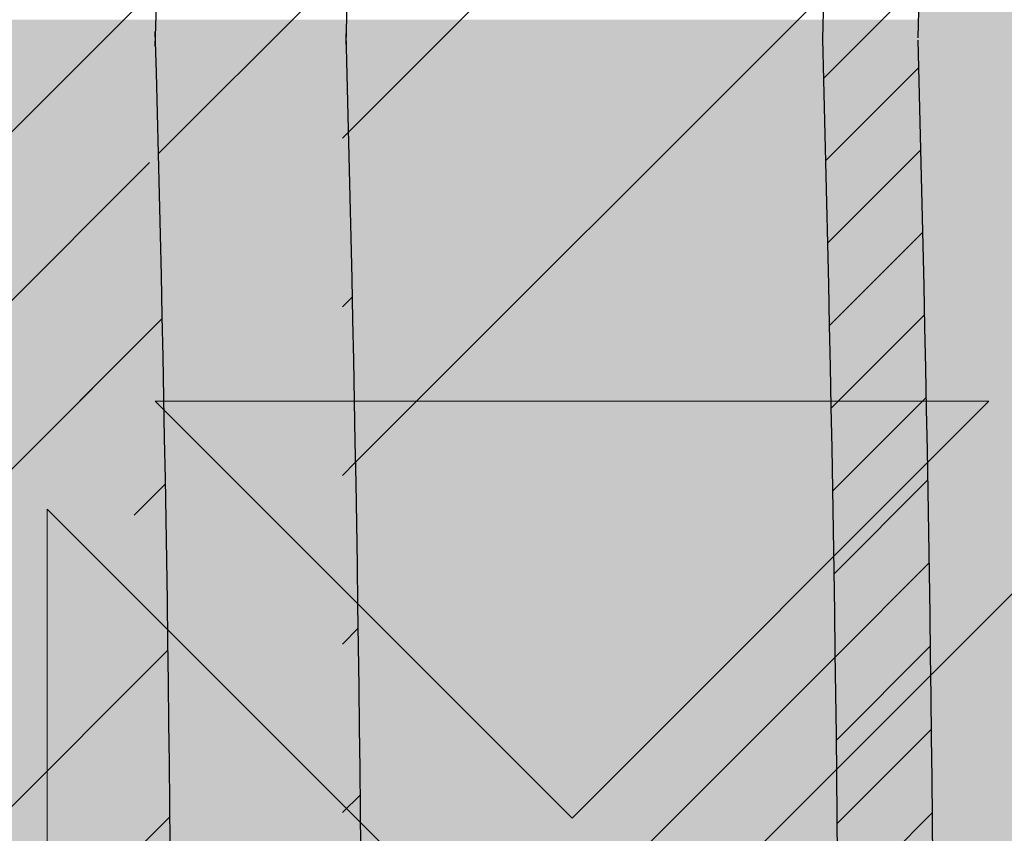
# Model space of a CAD drawing. Units: inches. Extents: x 844 to 2234, y 346 to 1084.
# Tile 11 of 93: x 1124.948 to 1126.594, y 694.861 to 696.22. Entities that reach past the tile are written whole.
import ezdxf

# ---------------------------------------------------------------- set-up
doc = ezdxf.new("R2010")
doc.units = ezdxf.units.IN
doc.header["$MEASUREMENT"] = 0
for name, color, linetype, lineweight in [('A-ANNO-DIMS', 2, 'Continuous', 18), ('furniture', 8, 'Continuous', 18), ('RA-AP-01$0$INT', 35, 'Continuous', 5)]:
    doc.layers.add(name, color=color, linetype=linetype, lineweight=lineweight)
doc.layers.add('RA-AP-01$0$FURN', color=3, linetype='Continuous')
doc.layers.add('RA-AP-01$0$WOOD', color=64, linetype='Continuous')
doc.styles.get("Standard").update_dxf_attribs({"font": 'arial.ttf'})
doc.dimstyles.get("Standard").update_dxf_attribs({"dimtxt": 6, "dimasz": 3, "dimexe": 0.18, "dimexo": 0.0625, "dimgap": 0.09, "dimtad": 0, "dimtih": 1, "dimtoh": 1, "dimdec": 1, "dimzin": 0, "dimdsep": 46, "dimlunit": 3, "dimtxsty": 'Standard', "dimblk": 'ARCHTICK', "dimcen": 0.09, "dimadec": 0, "dimazin": 0, "dimtfac": 1, "dimtdec": 1, "dimtofl": 0, "dimtmove": 0, "dimatfit": 3, "dimfxl": 1, "dimtolj": 1, "dimtzin": 0, "dimarcsym": 0})

# ---------------------------------------------------------------- blocks, each defined once
blk = doc.blocks.new('A$C18D01794')
at = {"layer": 'RA-AP-01$0$INT'}
h = blk.add_hatch(color=256, dxfattribs=at)
h.paths.add_polyline_path([(4.585917135068449, -6.356712009588271), (4.555206456959269, -6.35671200958746), (4.555206456959137, -6.387422687716308), (4.874495778835233, -6.706712009592356), (4.90520645695423, -6.676001331474049)])
h.paths.add_polyline_path([(5.255206456948813, -6.387422687716306), (5.255206456948682, -6.356712009605972), (5.224495778822613, -6.356712009605161), (4.905206456953498, -6.676001331474273), (4.935917135072151, -6.706712009592924)])
h.paths.add_polyline_path([(4.935917135072559, -6.706712009592068), (4.905206456953564, -6.737422687710376), (5.255206456951813, -7.087422687708613), (5.255206456951549, -7.026001331471008)])
h.paths.add_polyline_path([(4.555206456956399, -7.026001331471013), (4.555206456956134, -7.087422687708616), (4.905206456953821, -6.737422687710943), (4.874495778835166, -6.70671200959229)])
h = blk.add_hatch(color=256, dxfattribs=at)
h.paths.add_polyline_path([(4.585917135068448, -6.356712009588273), (4.614201406330596, -6.356712009589021), (4.668846067270487, -6.411356670531338), (4.723490728212344, -6.356712009591912), (4.771774999457151, -6.35671200959319), (4.826419660396886, -6.411356670535356), (4.862780050090322, -6.374996280843536), (4.844495778842715, -6.356712009595112), (4.862780050090411, -6.356712009595595), (4.905206456960182, -6.399138416468211), (4.947632863832445, -6.356712009597838), (4.965917135079675, -6.356712009598322), (4.947632863831759, -6.374996280845421), (4.983993253523576, -6.411356670538857), (5.038637914464627, -6.356712009600247), (5.08692218571208, -6.356712009601523), (5.141566846649976, -6.411356670541852), (5.196211507589851, -6.356712009604411), (5.224495778822615, -6.356712009605161), (4.905206456953975, -6.676001331473793)])
h.paths.add_polyline_path([(4.895206456956031, -6.637717060225675), (4.895206456958921, -6.528427738347902), (4.840561796018589, -6.583072399285802)], flags=16)
h.paths.add_polyline_path([(4.915206456955638, -6.637717060226121), (4.969851117895509, -6.583072399288678), (4.915206456957609, -6.528427738348344)], flags=16)
h.paths.add_polyline_path([(4.826419660395175, -6.568930263661755), (4.881064321335613, -6.514285602723745), (4.771774999456703, -6.514285602720857)], flags=16)
h.paths.add_polyline_path([(4.983993253519558, -6.568930263665262), (5.038637914460456, -6.514285602726792), (4.929348592581548, -6.514285602724816)], flags=16)
h.paths.add_polyline_path([(4.881064321336025, -6.494285602723742), (4.826419660397532, -6.439640941782821), (4.771774999457062, -6.494285602720859)], flags=16)
h.paths.add_polyline_path([(4.929348592582019, -6.494285602724817), (5.038637914460982, -6.494285602726792), (4.983993253522945, -6.439640941786327)], flags=16)
h.paths.add_polyline_path([(4.895206456960191, -6.480143467100443), (4.895206456962115, -6.407422687715913), (4.876922185715016, -6.389138416467584), (4.840561796021581, -6.425498806159401)], flags=16)
h.paths.add_polyline_path([(4.915206456958487, -6.480143467100889), (4.969851117899527, -6.425498806162279), (4.933490728206909, -6.389138416468043), (4.9152064569598, -6.40742268771434)], flags=16)
h.paths.add_polyline_path([(4.757632863832376, -6.480143467096812), (4.812277524772842, -6.425498806158772), (4.757632863834348, -6.370854145217844)], flags=16)
h.paths.add_polyline_path([(4.737632863832376, -6.480143467096286), (4.737632863834348, -6.370854145217375), (4.682988202893906, -6.425498806155385)], flags=16)
h.paths.add_polyline_path([(5.05278005008503, -6.480143467103376), (5.052780050087917, -6.370854145224413), (4.998135389146995, -6.425498806162908)], flags=16)
h.paths.add_polyline_path([(5.072780050085024, -6.480143467103744), (5.127424711025931, -6.42549880616527), (5.072780050087916, -6.370854145224832)], flags=16)
h.paths.add_polyline_path([(4.935917135072783, -6.706712009592292), (5.255206456948811, -6.387422687716309), (5.255206456948932, -6.415706958964177), (5.200561796010279, -6.470351619902839), (5.255206456949403, -6.524996280841948), (5.25520645694961, -6.5732805520894), (5.200561796009787, -6.627925213029239), (5.236922185702417, -6.664285602721864), (5.255206456949919, -6.646001331474357), (5.255206456949998, -6.664285602721898), (5.212780050078687, -6.706712009592262), (5.25520645695036, -6.749138416463932), (5.255206456950438, -6.767422687711313), (5.236922185702424, -6.749138416463297), (5.200561796009796, -6.785498806155928), (5.255206456950753, -6.840143467096874), (5.25520645695096, -6.888427738341682), (5.200561796010322, -6.943072399282328), (5.255206456951428, -6.997717060223427), (5.255206456951547, -7.026001331471006)])
h.paths.add_polyline_path([(5.042988202883395, -6.785498806155427), (5.097632863823085, -6.840143467095101), (5.097632863822622, -6.730854145216193)], flags=16)
h.paths.add_polyline_path([(5.028846067259663, -6.771356670531693), (5.083490728198774, -6.716712009592573), (4.974201406321001, -6.716712009593042)], flags=16)
h.paths.add_polyline_path([(5.117632863823087, -6.840143467095186), (5.172277524762331, -6.785498806155926), (5.11763286382262, -6.730854145216225)], flags=16)
h.paths.add_polyline_path([(5.08349072819877, -6.696712009593886), (5.028846067259652, -6.642067348654775), (4.974201406320998, -6.696712009593438)], flags=16)
h.paths.add_polyline_path([(5.131774999446817, -6.854285602718917), (5.186419660386065, -6.799640941779662), (5.241064321325782, -6.854285602719365)], flags=17)
h.paths.add_polyline_path([(5.131774999446228, -6.716712009592374), (5.186419660386065, -6.771356670532194), (5.222780050079488, -6.734996280838764), (5.204495778832781, -6.716712009592063)], flags=16)
h.paths.add_polyline_path([(5.097632863822613, -6.682569873970264), (5.097632863823061, -6.573280552091354), (5.042988202883383, -6.627925213031044)], flags=16)
h.paths.add_polyline_path([(5.131774999446899, -6.874285602718915), (5.241064321325809, -6.874285602719364), (5.186419660386591, -6.928930263658598)], flags=17)
h.paths.add_polyline_path([(5.131774999446226, -6.696712009594078), (5.204495778830767, -6.696712009594374), (5.22278005007868, -6.67842773834687), (5.186419660386049, -6.642067348654249)], flags=16)
h.paths.add_polyline_path([(5.11763286382262, -6.682569873970225), (5.17227752476232, -6.627925213030515), (5.117632863823064, -6.573280552091267)], flags=16)
h.paths.add_polyline_path([(5.186419660386069, -6.613783077405491), (5.241064321325754, -6.559138416465795), (5.131774999446791, -6.559138416466263)], flags=16)
h.paths.add_polyline_path([(5.131774999446872, -6.539138416466263), (5.24106432132578, -6.539138416465794), (5.186419660386554, -6.484493755526573)], flags=16)
h.paths.add_polyline_path([(5.255206456951811, -7.08742268770861), (5.255206456951895, -7.106712009588038), (4.555206456956052, -7.106712009588038), (4.555206456956136, -7.087422687708617), (4.905206456953973, -6.737422687710788)])
h.paths.add_polyline_path([(4.983993253513404, -6.8444937555241), (4.92934859257295, -6.899138416462108), (5.03863791445186, -6.899138416465014)], flags=16)
h.paths.add_polyline_path([(4.969851117889988, -6.83035161990006), (4.915206456952556, -6.775706958960171), (4.915206456949648, -6.884996280837944)], flags=16)
h.paths.add_polyline_path([(4.929348592572535, -6.919138416462105), (4.983993253511019, -6.973783077403037), (5.038637914451496, -6.919138416465012)], flags=16)
h.paths.add_polyline_path([(5.052780050074912, -6.93328055208906), (4.998135389134438, -6.987925213027088), (5.052780050072919, -7.042569873968025)], flags=16)
h.paths.add_polyline_path([(5.07278005007491, -6.933280552089588), (5.072780050072918, -7.042569873968497), (5.127424711013374, -6.987925213030498)], flags=16)
h.paths.add_polyline_path([(4.89520645695295, -6.775706958959721), (4.840561796013067, -6.830351619897157), (4.895206456950961, -6.884996280837494)], flags=16)
h.paths.add_polyline_path([(4.915206456948365, -6.933280552085403), (4.915206456946434, -7.006001331471951), (4.933490728192729, -7.024285602719066), (4.969851117886972, -6.987925213026453)], flags=16)
h.paths.add_polyline_path([(4.881064321327021, -6.899138416461022), (4.82641966038902, -6.84449375552057), (4.771774999448108, -6.899138416459029)], flags=16)
h.paths.add_polyline_path([(4.895206456950073, -6.933280552084951), (4.840561796009022, -6.987925213023558), (4.876922185700835, -7.024285602716997), (4.895206456948749, -7.006001331469487)], flags=16)
h.paths.add_polyline_path([(4.983993253510392, -7.0020673486505), (4.947632863816944, -7.038427738342319), (4.965917135064043, -7.05671200959023), (5.038637914448995, -7.056712009591555)], flags=16)
h.paths.add_polyline_path([(4.881064321326543, -6.91913841646102), (4.771774999447578, -6.919138416459031), (4.826419660385607, -6.973783077399508)], flags=16)
h.paths.add_polyline_path([(4.905206456946447, -7.014285602717636), (4.862780050074785, -7.056712009588352), (4.947632863816685, -7.056712009589775)], flags=16)
h.paths.add_polyline_path([(5.14156684663679, -7.002067348654549), (5.086922185696452, -7.056712009592438), (5.196211507574223, -7.056712009594425)], flags=16)
h.paths.add_polyline_path([(4.8264196603837, -7.002067348646972), (4.771774999442643, -7.056712009585575), (4.8444957788276, -7.056712009587508), (4.862780050075511, -7.038427738340416)], flags=16)
h.paths.add_polyline_path([(4.812277524760289, -6.98792521302292), (4.757632863822258, -6.933280552082447), (4.757632863819352, -7.042569873961408)], flags=16)
h.paths.add_polyline_path([(4.73763286382226, -6.933280552082079), (4.682988202881349, -6.987925213020536), (4.737632863819352, -7.04256987396099)], flags=16)
h.paths.add_polyline_path([(4.723490728195188, -7.056712009584289), (4.668846067257299, -7.002067348643949), (4.614201406317417, -7.056712009581383)], flags=16)
h.paths.add_polyline_path([(4.597632863829262, -6.706712009592262), (4.555206456957951, -6.664285602721896), (4.555206456958029, -6.646001331474357), (4.573490728205535, -6.664285602721864), (4.609851117898167, -6.627925213029238), (4.555206456958338, -6.573280552089402), (4.555206456958546, -6.524996280841952), (4.60985111789767, -6.470351619902839), (4.555206456959015, -6.415706958964177), (4.555206456959138, -6.387422687716309), (4.874495778835167, -6.70671200959229), (4.5552064569564, -7.026001331471015), (4.555206456956523, -6.997717060223433), (4.609851117897629, -6.94307239928233), (4.555206456956988, -6.888427738341681), (4.555206456957198, -6.840143467096881), (4.609851117898153, -6.78549880615593), (4.573490728205528, -6.749138416463297), (4.555206456957507, -6.76742268771132), (4.555206456957585, -6.749138416463933)])
h.paths.add_polyline_path([(4.712780050085332, -6.730854145216195), (4.712780050084863, -6.840143467095105), (4.767424711024555, -6.785498806155427)], flags=16)
h.paths.add_polyline_path([(4.726922185709173, -6.716712009592573), (4.781566846648288, -6.771356670531693), (4.836211507586949, -6.716712009593043)], flags=16)
h.paths.add_polyline_path([(4.692780050085327, -6.730854145216225), (4.638135389145619, -6.785498806155928), (4.692780050084865, -6.840143467095185)], flags=16)
h.paths.add_polyline_path([(4.726922185709182, -6.696712009593886), (4.836211507586949, -6.696712009593436), (4.7815668466483, -6.642067348654773)], flags=16)
h.paths.add_polyline_path([(4.678637914461726, -6.71671200959237), (4.605917135075169, -6.716712009592063), (4.587632863828464, -6.734996280838766), (4.623993253521887, -6.771356670532195)], flags=16)
h.paths.add_polyline_path([(4.712780050085336, -6.68256987397026), (4.767424711024568, -6.627925213031042), (4.71278005008489, -6.573280552091352)], flags=16)
h.paths.add_polyline_path([(4.678637914461726, -6.696712009594076), (4.623993253521899, -6.642067348654247), (4.587632863829271, -6.67842773834687), (4.605917135077185, -6.696712009594376)], flags=16)
h.paths.add_polyline_path([(4.692780050085336, -6.682569873970228), (4.692780050084889, -6.573280552091267), (4.638135389145632, -6.627925213030515)], flags=16)
h.paths.add_polyline_path([(4.623993253521885, -6.799640941779662), (4.678637914461131, -6.854285602718915), (4.56934859258217, -6.854285602719365)], flags=17)
h.paths.add_polyline_path([(4.623993253521901, -6.613783077405509), (4.678637914461158, -6.559138416466263), (4.569348592582195, -6.559138416465795)], flags=16)
h.paths.add_polyline_path([(4.678637914461051, -6.874285602718915), (4.623993253521361, -6.928930263658598), (4.569348592582143, -6.874285602719364)], flags=17)
h.paths.add_polyline_path([(4.678637914461076, -6.539138416466263), (4.623993253521399, -6.484493755526573), (4.569348592582167, -6.539138416465796)], flags=16)
h = blk.add_hatch(color=256, dxfattribs=at)
h.paths.add_polyline_path([(4.895206456952951, -6.77570695895972), (4.840561796013068, -6.830351619897156), (4.895206456950958, -6.884996280837495)])
h.paths.add_polyline_path([(4.915206456949649, -6.884996280837942), (4.969851117889987, -6.830351619900054), (4.915206456952556, -6.775706958960171)])
h.paths.add_polyline_path([(5.038637914451862, -6.899138416465013), (4.983993253513403, -6.8444937555241), (4.929348592572953, -6.899138416462106)])
h.paths.add_polyline_path([(4.929348592572535, -6.919138416462105), (4.983993253511018, -6.973783077403037), (5.038637914451497, -6.919138416465012)])
h.paths.add_polyline_path([(4.915206456948366, -6.933280552085397), (4.915206456946433, -7.006001331471951), (4.93349072819273, -7.024285602719068), (4.969851117886972, -6.987925213026454)])
h.paths.add_polyline_path([(5.038637914448995, -7.056712009591553), (4.983993253510389, -7.002067348650502), (4.947632863816946, -7.038427738342318), (4.965917135064043, -7.05671200959023)])
h.paths.add_polyline_path([(5.05278005007292, -7.042569873968023), (5.05278005007491, -6.933280552089059), (4.998135389134438, -6.987925213027088)])
h.paths.add_polyline_path([(5.07278005007292, -7.042569873968496), (5.127424711013374, -6.987925213030498), (5.072780050074909, -6.933280552089588)])
h.paths.add_polyline_path([(5.141566846636789, -7.002067348654547), (5.086922185696449, -7.056712009592438), (5.196211507574223, -7.056712009594425)])
h.paths.add_polyline_path([(4.947632863816688, -7.056712009589774), (4.905206456946449, -7.014285602717634), (4.862780050074784, -7.056712009588353)])
h.paths.add_polyline_path([(4.840561796009025, -6.987925213023556), (4.876922185700834, -7.024285602716997), (4.895206456948747, -7.006001331469488), (4.895206456950075, -6.933280552084953)])
h.paths.add_polyline_path([(4.88106432132654, -6.919138416461021), (4.771774999447577, -6.919138416459031), (4.826419660385606, -6.973783077399508)])
h.paths.add_polyline_path([(4.881064321327019, -6.899138416461022), (4.826419660389019, -6.844493755520571), (4.771774999448108, -6.89913841645903)])
h.paths.add_polyline_path([(4.757632863819352, -7.042569873961409), (4.812277524760284, -6.987925213022922), (4.757632863822259, -6.933280552082447)])
h.paths.add_polyline_path([(4.8264196603837, -7.002067348646974), (4.771774999442646, -7.056712009585575), (4.844495778827599, -7.05671200958751), (4.862780050075512, -7.038427738340417)])
h.paths.add_polyline_path([(4.737632863819352, -7.042569873960988), (4.737632863822258, -6.933280552082078), (4.682988202881349, -6.987925213020538)])
h.paths.add_polyline_path([(4.668846067257299, -7.002067348643952), (4.61420140631742, -7.056712009581384), (4.723490728195189, -7.056712009584292)])
for p, q in [((4.905206456953975, -6.737422687710788), (5.255206456951811, -7.087422687708611)), ((5.07278005007491, -6.933280552089588), (5.07278005007292, -7.042569873968497)), ((5.07278005007292, -7.042569873968497), (5.127424711013374, -6.987925213030498)), ((5.086922185696454, -7.056712009592434), (5.141566846636789, -7.002067348654547)), ((5.196211507574223, -7.056712009594425), (5.141566846636789, -7.002067348654547)), ((5.086922185696452, -7.056712009592438), (5.196211507574223, -7.056712009594425))]:
    blk.add_line(p, q, dxfattribs=at)
blk = doc.blocks.new('A$C32926AE1')
at = {"layer": 'RA-AP-01$0$FURN'}
h = blk.add_hatch(dxfattribs=at)
h.set_pattern_fill('ANSI31', color=256, scale=0.1, style=0)
h.set_pattern_definition([(45, (0, 0), (-0.0088388347648318, 0.0088388347648318), [])])
edge = h.paths.add_edge_path(flags=16)
edge.add_arc((4.904771284329206, 4.246793130718756), 0.2603971832811541, 75.22398030683196, 104.7760196931204)
edge.add_arc((4.904771284329206, 4.246793130718756), 0.2603971832811541, 75.223980306832, 104.77601969312039, ccw=False)
edge = h.paths.add_edge_path(flags=16)
edge.add_arc((4.904771284329206, 4.067062675376612), 0.2603971832811541, 255.2239803068796, 284.776019693168)
edge.add_arc((4.904771284329206, 4.067062675376612), 0.2603971832811541, 255.22398030687958, 284.77601969316805, ccw=False)
edge = h.paths.add_edge_path(flags=0)
edge.add_arc((4.904771284329206, 4.067062675376612), 0.2603971832811541, 255.2239803068796, 284.776019693168)
edge.add_arc((4.904771284329206, 4.067062675376612), 0.2603971832811541, 255.22398030687958, 284.77601969316805, ccw=False)
edge = h.paths.add_edge_path(flags=0)
edge.add_arc((4.904771284329206, 4.067062675376612), 0.2603971832811541, 255.2239803068796, 284.776019693168)
edge.add_arc((4.904771284329206, 4.067062675376612), 0.2603971832811541, 255.22398030687958, 284.77601969316805, ccw=False)
edge = h.paths.add_edge_path()
edge.add_arc((4.604388392048174, 4.588829985554312), 0.1599999999999918, 342.3781640246255, 354.4317409793762)
edge.add_arc((5.090145208887507, 4.43216705527679), 0.3503971832811637, 162.0091218307731, 180.3186872093483)
edge.add_arc((5.205154176610243, 4.588829985554953), 0.1599999999999917, 185.5682590208461, 197.6218359767349)
edge.add_arc((4.904771284329229, 4.246793130718735), 0.3503971832811761, 72.00912183053516, 107.9908781690354)
edge.add_arc((9.535952835716557, 4.28682295566602), 4.798342501046485, 178.2875002453811, 181.5576802719453)
edge.add_arc((4.719397359771122, 4.43216705527679), 0.3503971832811637, 359.6813127906516, 377.9908781692269)
edge.add_arc((9.535967292294904, 4.286822350292874), 4.778371420254705, 178.2965938931842, 181.5667745797229)
edge.add_arc((4.719397359771122, 4.43216705527679), 0.3303971832811637, 359.6813127906516, 377.9908781692269)
edge.add_arc((0.2735752763637294, 4.286822350292874), 4.7783714202547, 358.4332254202771, 361.7034061068158)
edge.add_arc((5.061434214606998, 4.732549947558029), 0.1600000000000254, 252.3781640250584, 264.4317409792362)
edge.add_arc((4.748108354051257, 4.732549947558012), 0.1600000000000541, 275.5682590208426, 287.6218359759532)
edge.add_arc((4.604388392048115, 4.588829985554317), 0.1800000000000505, 342.3567572500182, 349.3735009646207)
edge.add_arc((5.205154176610254, 4.588829985554976), 0.1800000000000069, 190.6264990356027, 197.6432427513933)
edge.add_arc((5.061434214607106, 4.732549947558013), 0.1800000000000424, 252.3567572496606, 259.3735009644582)
edge.add_arc((4.904771284329208, 4.246793130718737), 0.3303971832811676, 71.99844483668534, 108.0015551637021)
edge.add_arc((4.748108354051414, 4.732549947558045), 0.1800000000000547, 280.6264990355479, 287.6432427495938)
edge.add_arc((5.090145208887514, 4.432167055276789), 0.2803971832811691, 162.8706300666893, 180.816523289902)
edge.add_arc((4.719397359771136, 4.432167055276689), 0.2803971832811534, 359.183476710103, 377.1293699333214)
edge.add_arc((4.904771284329222, 4.246793130718737), 0.2803971832811769, 72.87063006672916, 107.1293699332334)
edge.add_arc((5.090145208887522, 4.432167055276788), 0.2603971832811776, 165.2239803068007, 180.9953123810312)
edge.add_arc((4.719397359771141, 4.432167055276699), 0.2603971832811458, 359.0046876189768, 374.7760196932087)
edge.add_arc((5.090145208887507, 4.43216705527679), 0.3303971832811637, 162.0091218307731, 180.3186872093483)
edge.add_arc((9.53595427642584, 4.285015535491528), 4.728345371032053, 178.265043920078, 181.5679956281801)
edge.add_arc((0.2735882922327999, 4.285015535491582), 4.728345371032045, 358.4320043718193, 361.7349560799204)
edge.add_arc((9.535953591267507, 4.284458026472751), 4.708343996644348, 178.2573054306777, 181.5704995759608)
edge.add_arc((0.273588977391114, 4.284458026472785), 4.708343996644358, 358.4295004240388, 361.7426945693213)
edge.add_arc((0.2735889773911131, 4.029397779622582), 4.708343996644359, 358.2573054306787, 361.5704995759613)
edge.add_arc((9.535953591267518, 4.029397779622618), 4.708343996644359, 178.4295004240391, 181.7426945693223)
edge.add_arc((0.2735882922327901, 4.028840270603786), 4.728345371032054, 358.2650439200796, 361.5679956281808)
edge.add_arc((9.53595427642584, 4.028840270603841), 4.728345371032054, 178.4320043718199, 181.7349560799219)
edge.add_arc((0.2735752763637302, 4.027033455802493), 4.778371420254699, 358.2965938931842, 361.5667745797229)
edge.add_arc((4.719397359771122, 3.881688750818578), 0.3303971832811637, 342.0091218307731, 360.3186872093484)
edge.add_arc((5.090145208887507, 3.881688750818578), 0.3303971832811637, 179.6813127906516, 197.9908781692269)
edge.add_arc((9.535967292294904, 4.027033455802493), 4.778371420254705, 178.433225420277, 181.7034061068158)
edge.add_arc((4.719397359771122, 3.881688750818578), 0.3503971832811637, 342.0091218307731, 360.3186872093484)
edge.add_arc((9.53595283571655, 4.027032850429349), 4.79834250104648, 178.4423197280546, 181.7124997546188)
edge.add_arc((4.719397359771141, 3.881688750818669), 0.2603971832811458, 345.2239803067913, 360.9953123810232)
edge.add_arc((5.090145208887522, 3.88168875081858), 0.2603971832811776, 179.0046876189687, 194.7760196931993)
edge.add_arc((4.904771284329222, 4.067062675376631), 0.2803971832811769, 252.8706300667665, 287.1293699332708)
edge.add_arc((4.719397359771136, 3.881688750818678), 0.2803971832811534, 342.8706300666787, 360.8165232898969)
edge.add_arc((5.090145208887514, 3.881688750818579), 0.2803971832811691, 179.183476710098, 197.1293699333106)
edge.add_arc((4.748108354051414, 3.581305858537323), 0.1800000000000547, 72.3567572504062, 79.37350096445199)
edge.add_arc((4.904771284329208, 4.067062675376631), 0.3303971832811676, 251.9984448362979, 288.0015551633146)
edge.add_arc((5.061434214607106, 3.581305858537355), 0.1800000000000424, 100.6264990355418, 107.6432427503394)
edge.add_arc((5.205154176610254, 3.725025820540392), 0.1800000000000069, 162.3567572486066, 169.3735009643972)
edge.add_arc((4.604388392048115, 3.725025820541051), 0.1800000000000505, 10.62649903537925, 17.64324274998182)
edge.add_arc((4.748108354051257, 3.581305858537356), 0.1600000000000541, 72.37816402404681, 84.43174097915735)
edge.add_arc((4.904771284329229, 4.067062675376632), 0.3503971832811761, 252.0091218309645, 287.9908781694648)
edge.add_arc((5.061434214606998, 3.581305858537339), 0.1600000000000254, 95.56825902076373, 107.6218359749416)
edge.add_arc((5.205154176610243, 3.725025820540414), 0.1599999999999917, 162.3781640232651, 174.4317409791539)
edge.add_arc((5.090145208887507, 3.881688750818578), 0.3503971832811637, 179.6813127906516, 197.9908781692269)
edge.add_arc((4.604388392048174, 3.725025820541056), 0.1599999999999918, 5.568259020623824, 17.62183597537444)
edge.add_arc((0.2735897329420762, 4.28682295566602), 4.798342501046482, 358.4423197280547, 361.7124997546188)
edge.add_arc((0.2735897329420691, 4.027032850429348), 4.798342501046489, 358.2875002453812, 361.5576802719453)
at = {"layer": 'RA-AP-01$0$WOOD'}
h = blk.add_hatch(color=256, dxfattribs=at)
h.dxf.hatch_style = 1
h.paths.add_polyline_path([(5.157430609644524, 4.573483066760929, -0.1009492694046607), (5.155401577623758, 4.593365984175333, -0.1842662638101597), (5.172249623284174, 4.638795604568598, 0.2056608120311276), (5.179560981299304, 4.661316324430096, 0.3614336704623542), (5.134352340494423, 4.706524965234944, 0.2056608120311297), (5.111831620632933, 4.699213607219793, -0.1842662638101113), (5.066402000239693, 4.682365561559342, -0.1055311479399994), (5.045656153913092, 4.68467289944697, 0.1567636581983829), (4.763886414745334, 4.684672899446966, -0.1055311479399895), (4.743140568418733, 4.68236556155934, -0.1842662638100833), (4.6977109480255, 4.69921360721979, 0.2056608120302612), (4.675190228164109, 4.706524965234949, 0.3614336704708441), (4.629981587358889, 4.66131632442871, 0.2056608120245944), (4.637292945374126, 4.638795604567974, -0.1842662638101024), (4.654140991034615, 4.59336598417475, -0.1009492694055169), (4.652111959013835, 4.573483066760181, 0.021410119221476), (4.629748025606143, 4.156712009541676, 0.0214101192214795), (4.652111959013809, 3.739940952323101, -0.1009492694059586), (4.654140991034615, 3.720058034908448, -0.1842662638100975), (4.637292945374126, 3.674628414515226, 0.2056608120245705), (4.629981587358889, 3.652107694654492, 0.3614336704708879), (4.675190228164113, 3.606899053848249, 0.2056608120302384), (4.697710948025501, 3.614210411863408, -0.1842662638100995), (4.743140568418738, 3.63105845752386, -0.1055311479402541), (4.763886414745388, 3.628751119636215, 0.1567636581983776), (5.045656153913137, 3.628751119636244, -0.1055311479397538), (5.066402000239692, 3.631058457523857, -0.1842662638101067), (5.111831620632931, 3.614210411863407, 0.2056608120310924), (5.134352340494417, 3.606899053848256, 0.3614336704624001), (5.179560981299307, 3.652107694653103, 0.2056608120311314), (5.172249623284175, 3.6746284145146, -0.1842662638101402), (5.155401577623758, 3.72005803490786, -0.1009492694051366), (5.15743060964455, 3.739940952322354, 0.0214101192215073), (5.179794543052287, 4.156712009541468, 0.0214101192215252)])
h.paths.add_polyline_path([(4.639748609479751, 4.156712009541513, 0.0213537860821624), (4.661970494867118, 3.741887061152232, -0.094075836301374), (4.664143710413708, 3.7196126951003, -0.1824818158568985), (4.644813765429836, 3.668037719127816, 0.2056608120245319), (4.639939526753007, 3.653023905887301, 0.3614336704710246), (4.676106439397173, 3.616856993242342, 0.2056608120302234), (4.691120252638095, 3.621731231919122, -0.1824818158602558), (4.742695228611606, 3.641061176902986, -0.1029891339458722), (4.766991894714349, 3.638256818950944, 0.156709409989566), (5.042550673941472, 3.638256818950105, -0.102989133958497), (5.066847340047078, 3.641061176902949, -0.1824818158594995), (5.118422316020358, 3.621731231919103, 0.2056608120311416), (5.133436129261316, 3.616856993242346, 0.3614336704621468), (5.169603041905217, 3.653023905886178, 0.2056608120310986), (5.164728803228477, 3.668037719127177, -0.1824818158565612), (5.145398858244737, 3.719612695099578, -0.0940758363009313), (5.147572073791232, 3.741887061151398, 0.0213537860822023), (5.169793959178681, 4.156712009541451, 0.0213537860822226), (5.147572073791203, 4.571536957931898, -0.0940758363005034), (5.145398858244737, 4.59381132398362, -0.1824818158565587), (5.164728803228476, 4.645386299956021, 0.2056608120311045), (5.169603041905216, 4.66040011319702, 0.3614336704621845), (5.133436129261313, 4.696567025840856, 0.2056608120310773), (5.118422316020359, 4.691692787164098, -0.182481815859508), (5.066847340047078, 4.67236284218025, -0.1029891339584606), (5.04255067394148, 4.675167200133092, 0.156709409989566), (4.766991894714357, 4.675167200132257, -0.1029891339458842), (4.742695228611611, 4.672362842180213, -0.1824818158602725), (4.691120252638095, 4.691692787164077, 0.2056608120302152), (4.676106439397174, 4.696567025840858, 0.3614336704710363), (4.639939526753005, 4.660400113195899, 0.2056608120245495), (4.644813765429837, 4.645386299955384, -0.1824818158568934), (4.664143710413708, 4.593811323982902, -0.0940758363009187), (4.661970494867149, 4.571536957931074, 0.021353786082177)], flags=16)
h.paths.add_polyline_path([(5.129794543052235, 4.432167055276933, -0.0141661062790638), (5.130152669293814, 4.156927903047693, -0.0141661062790647), (5.129794543052234, 3.881688750818433, -0.0785247771143638), (5.10979738006795, 3.755143611847103, 0.0945969212073497), (5.105408519571111, 3.717898134952927, 0.1043170707844957), (5.116074640131521, 3.670385395016088, 0.1043170707864965), (5.068561900193738, 3.681051515576561, 0.09459692119553), (5.031316423304057, 3.676662655080835, -0.1580239521427272), (4.778226145355827, 3.676662655080367, 0.0945969211986668), (4.740980668464973, 3.681051515576592, 0.1043170707882822), (4.693467928526415, 3.670385395015844, 0.1043170707867916), (4.704134049087309, 3.717898134953662, 0.0945969211972894), (4.69974518859162, 3.755143611844042, -0.0785247771163196), (4.679748025606343, 3.881688750818406, -0.0141661062790663), (4.679389899364763, 4.156927903047693, -0.0141661062790672), (4.679748025606343, 4.432167055276998, -0.0785247771163064), (4.699745188591625, 4.55871219425134, 0.094596921197333), (4.704134049087308, 4.595957671141738, 0.1043170707867205), (4.693467928526416, 4.643470411079523, 0.1043170707882628), (4.740980668464965, 4.632804290518776, 0.0945969211988114), (4.778226145355874, 4.637193151015016, -0.158023952142669), (5.031316423304015, 4.637193151014546, 0.0945969211956361), (5.068561900193736, 4.632804290518806, 0.1043170707864979), (5.11607464013152, 4.643470411079278, 0.1043170707844617), (5.105408519571112, 4.595957671142455, 0.0945969212074597), (5.109797380067959, 4.558712194248236, -0.0785247771143467)], flags=0)
h.paths.add_polyline_path([(5.119794532311105, 4.432259799204851, -0.0142000800617244), (5.120156169157484, 4.156927903047701, -0.0142000800617277), (5.119794532311105, 3.881596006890482, -0.0784894509520253), (5.100273383573699, 3.758192358677797, 0.0940138827242913), (5.095413455884425, 3.717477693979438, 0.0606271852308753), (5.099615656341024, 3.686844378806616, 0.0606271852322524), (5.068982341167493, 3.691046579263239, 0.0940138827010453), (5.028267676478798, 3.686186651576848, -0.1580706864508061), (4.781274892180912, 3.686186651576435, 0.0940138827026903), (4.740560227491556, 3.691046579263279, 0.0606271852339895), (4.709926912317155, 3.686844378806508, 0.0606271852329405), (4.714129112773991, 3.717477693980356, 0.094013882701304), (4.709269185087677, 3.758192358669163, -0.0784894509577193), (4.689748036347473, 3.881596006890469, -0.014200080061729), (4.689386399501094, 4.156927903047709, -0.0142000800617217), (4.689748036347473, 4.432259799204808, -0.078489450957724), (4.709269185087651, 4.555663447426125, 0.0940138827014585), (4.714129112773992, 4.596378112114996, 0.0606271852329731), (4.709926912317154, 4.62701142728886, 0.0606271852340196), (4.74056022749157, 4.622809226832087, 0.0940138827024997), (4.781274892180847, 4.627669154518912, -0.1580706864508359), (5.028267676478777, 4.627669154518526, 0.0940138827010946), (5.068982341167492, 4.622809226832129, 0.060627185232254), (5.099615656341024, 4.627011427288751, 0.0606271852308727), (5.095413455884425, 4.59637811211593, 0.0940138827241088), (5.100273383573675, 4.555663447417647, -0.0784894509520978)], flags=0)
h.paths.add_polyline_path([(5.06978912287499, 4.430218106756144, -0.014241683694547), (5.070173729147532, 4.156927903047672, -0.0142416836945458), (5.06978912287499, 3.883637699339223, -0.0800609523125196), (5.052662118612511, 3.773463122773442, 0.0526421978001116), (5.04590916754064, 3.740550867606997, 0.0526421977992423), (5.012996912374707, 3.73379791653534, -0.1583028414718258), (4.796545656286308, 3.73379791653451, 0.0526421978034211), (4.763633401117837, 3.740550867607021, 0.0526421978018622), (4.756880450045755, 3.773463122774558, -0.0800609523117106), (4.739753445783639, 3.883637699339268, -0.0142416836945435), (4.739368839511098, 4.156927903047671, -0.0142416836945477), (4.739753445783639, 4.430218106756155, -0.0800609523116345), (4.75688045004574, 4.540392683320762, 0.052642197801941), (4.763633401117837, 4.573304938488346, 0.0526421978035071), (4.796545656286361, 4.580057889560873, -0.1583028414717561), (5.012996912374669, 4.580057889560039, 0.0526421977993048), (5.04590916754064, 4.57330493848837, 0.0526421978002057), (5.052662118612529, 4.540392683321868, -0.080060952312477)], flags=0)
h.paths.add_polyline_path([(5.049789715110557, 4.43038092723357, -0.0143097550741839), (5.05018085590259, 4.156927903047715, -0.0143097550741854), (5.049789715110558, 3.883474878861827, -0.0800685599149176), (5.03362098255317, 3.779581877367999, 0.0306258898956367), (5.028241146483733, 3.758218888663947, 0.0306258898977031), (5.006878157778253, 3.75283905259408, -0.1583983521624096), (4.802664410878162, 3.752839052594731, 0.0306258898946014), (4.781301422174808, 3.758218888663924, 0.0306258898967912), (4.775921586105202, 3.779581877368794, -0.080068559914251), (4.759752853548071, 3.883474878861786, -0.0143097550741854), (4.759361712756037, 4.156927903047671, -0.0143097550741854), (4.759752853548071, 4.430380927233557, -0.0800685599142479), (4.775921586105193, 4.534273928726546, 0.0306258898968306), (4.781301422174808, 4.555636917431444, 0.0306258898945754), (4.802664410878143, 4.561016753500631, -0.1583983521624168), (5.006878157778244, 4.561016753501291, 0.0306258898977177), (5.028241146483733, 4.555636917431421, 0.0306258898958182), (5.03362098255321, 4.534273928727244, -0.080068559914796)], flags=0)
h.paths.add_polyline_path([(4.999766070382627, 4.428171244713864, -0.0143443147609634), (5.000198441819402, 4.156927903047689, -0.0143443147609612), (4.999766070382627, 3.885684561381556, -0.0784641635803329), (4.987356730658798, 3.799103304488872, -0.1506053783831347), (4.822185837999821, 3.79910330448882, -0.0784641635803318), (4.809776498276007, 3.885684561381509, -0.014344314760963), (4.809344126839227, 4.156927903047677, -0.0143443147609645), (4.809776498276007, 4.428171244713873, -0.0784641635803192), (4.822185837999822, 4.514752501606549, -0.1506053783831338), (4.987356730658798, 4.514752501606494, -0.078464163580285)], flags=0)
h.paths.add_polyline_path([(4.979755254238824, 4.42764379880488, -0.0143772539198268), (4.980205517789977, 4.156927903047693, -0.0143772539198275), (4.979755254238824, 3.886212007290489, -0.0689242507424422), (4.971183264704897, 3.815276770442801, -0.1296645318904179), (4.838359303953726, 3.815276770442746, -0.0689242507424186), (4.829787314419809, 3.886212007290419, -0.0143772539198292), (4.829337050868653, 4.156927903047653, -0.0143772539198325), (4.829787314419809, 4.427643798804946, -0.0689242507424211), (4.838359303953725, 4.498579035652621, -0.1296645318904187), (4.971183264704897, 4.498579035652565, -0.0689242507424401)], flags=0)
h = blk.add_hatch(color=256, dxfattribs=at)
h.dxf.hatch_style = 1
h.paths.add_polyline_path([(5.145398858244737, 4.59381132398362, -0.1824818158565616), (5.164728803228476, 4.645386299956021, 0.2056608120311045), (5.169603041905216, 4.66040011319702, 0.3614336704621845), (5.133436129261313, 4.696567025840856, 0.2056608120310773), (5.118422316020359, 4.691692787164098, -0.182481815859508), (5.066847340047078, 4.67236284218025, -0.1029891339584606), (5.04255067394148, 4.675167200133092, 0.156709409989566), (4.766991894714357, 4.675167200132257, -0.1029891339458842), (4.742695228611611, 4.672362842180213, -0.1824818158602725), (4.691120252638095, 4.691692787164077, 0.2056608120302152), (4.676106439397174, 4.696567025840858, 0.3614336704710363), (4.639939526753005, 4.660400113195899, 0.2056608120245495), (4.644813765429837, 4.645386299955384, -0.1824818158568934), (4.664143710413708, 4.593811323982902, -0.0940758363009187), (4.661970494867149, 4.571536957931074, 0.0213537860821772), (4.639748609479751, 4.156712009541507, 0.0213537860821625), (4.661970494867119, 3.741887061152226, -0.0940758363013071), (4.664143710413708, 3.719612695100309, -0.1824818158569294), (4.644813765429836, 3.668037719127816, 0.2056608120245319), (4.639939526753007, 3.653023905887301, 0.3614336704710246), (4.676106439397173, 3.616856993242342, 0.2056608120302234), (4.691120252638095, 3.621731231919122, -0.1824818158602558), (4.742695228611606, 3.641061176902986, -0.1029891339458722), (4.766991894714349, 3.638256818950944, 0.156709409989566), (5.042550673941472, 3.638256818950105, -0.102989133958497), (5.066847340047078, 3.641061176902949, -0.1824818158594995), (5.118422316020358, 3.621731231919103, 0.2056608120311416), (5.133436129261316, 3.616856993242346, 0.3614336704621468), (5.169603041905217, 3.653023905886178, 0.2056608120310986), (5.164728803228477, 3.668037719127177, -0.1824818158565612), (5.145398858244737, 3.719612695099578, -0.0940758363009313), (5.147572073791232, 3.741887061151398, 0.0213537860822023), (5.169793959178681, 4.156712009541451, 0.0213537860822226), (5.147572073791203, 4.571536957931898, -0.0940758363004996)])
h.paths.add_polyline_path([(5.109797380067958, 4.55871219424824, -0.0785247771143472), (5.129794543052234, 4.432167055276936, -0.0141661062790644), (5.130152669293814, 4.156927903047685, -0.014166106279066), (5.129794543052234, 3.881688750818401, -0.0785247771143517), (5.109797380067946, 3.755143611847092, 0.0945969212073132), (5.105408519571111, 3.717898134952929, 0.1043170707844995), (5.116074640131521, 3.670385395016088, 0.1043170707864965), (5.068561900193738, 3.681051515576561, 0.09459692119553), (5.031316423304057, 3.676662655080835, -0.1580239521427272), (4.778226145355827, 3.676662655080367, 0.0945969211986668), (4.740980668464973, 3.681051515576592, 0.1043170707882822), (4.693467928526415, 3.670385395015844, 0.1043170707867916), (4.704134049087309, 3.717898134953662, 0.0945969211972894), (4.69974518859162, 3.755143611844042, -0.0785247771163196), (4.679748025606343, 3.881688750818406, -0.0141661062790663), (4.679389899364763, 4.156927903047693, -0.0141661062790672), (4.679748025606343, 4.432167055276998, -0.0785247771163064), (4.699745188591625, 4.55871219425134, 0.094596921197333), (4.704134049087308, 4.595957671141738, 0.1043170707867205), (4.693467928526416, 4.643470411079523, 0.1043170707882628), (4.740980668464965, 4.632804290518776, 0.0945969211988114), (4.778226145355874, 4.637193151015016, -0.158023952142669), (5.031316423304015, 4.637193151014546, 0.0945969211956361), (5.068561900193736, 4.632804290518806, 0.1043170707864979), (5.11607464013152, 4.643470411079278, 0.1043170707844617), (5.105408519571112, 4.595957671142455, 0.0945969212074504)], flags=16)
h.paths.add_polyline_path([(5.100273383573655, 4.55566344741771, -0.0784894509521388), (5.119794532311105, 4.432259799204852, -0.0142000800617252), (5.120156169157484, 4.156927903047686, -0.014200080061726), (5.119794532311105, 3.881596006890502, -0.0784894509520446), (5.100273383573696, 3.758192358677786, 0.0940138827242721), (5.095413455884425, 3.717477693979436, 0.0606271852308692), (5.099615656341024, 3.686844378806616, 0.0606271852322522), (5.068982341167493, 3.691046579263239, 0.0940138827010453), (5.028267676478798, 3.686186651576848, -0.1580706864508061), (4.781274892180912, 3.686186651576435, 0.0940138827026903), (4.740560227491556, 3.691046579263279, 0.0606271852339895), (4.709926912317155, 3.686844378806508, 0.0606271852329405), (4.714129112773991, 3.717477693980356, 0.094013882701304), (4.709269185087677, 3.758192358669163, -0.0784894509577193), (4.689748036347473, 3.881596006890469, -0.014200080061729), (4.689386399501094, 4.156927903047709, -0.0142000800617217), (4.689748036347473, 4.432259799204808, -0.078489450957724), (4.709269185087651, 4.555663447426125, 0.0940138827014585), (4.714129112773992, 4.596378112114996, 0.0606271852329731), (4.709926912317154, 4.62701142728886, 0.0606271852340196), (4.74056022749157, 4.622809226832087, 0.0940138827024997), (4.781274892180847, 4.627669154518912, -0.1580706864508359), (5.028267676478777, 4.627669154518526, 0.0940138827010946), (5.068982341167492, 4.622809226832129, 0.060627185232254), (5.099615656341024, 4.627011427288751, 0.0606271852308727), (5.095413455884425, 4.59637811211593, 0.094013882723957)], flags=0)
h.paths.add_polyline_path([(5.04590916754064, 4.57330493848837, 0.0526421978002057), (5.052662118612529, 4.540392683321868, -0.0800609523124783), (5.06978912287499, 4.430218106756142, -0.0142416836945469), (5.070173729147532, 4.156927903047672, -0.0142416836945458), (5.06978912287499, 3.883637699339223, -0.0800609523125196), (5.052662118612511, 3.773463122773442, 0.0526421978001116), (5.04590916754064, 3.740550867606997, 0.0526421977992423), (5.012996912374707, 3.73379791653534, -0.1583028414718258), (4.796545656286308, 3.73379791653451, 0.0526421978034211), (4.763633401117837, 3.740550867607021, 0.0526421978018622), (4.756880450045755, 3.773463122774558, -0.0800609523117106), (4.739753445783639, 3.883637699339268, -0.0142416836945435), (4.739368839511098, 4.156927903047671, -0.0142416836945477), (4.739753445783639, 4.430218106756155, -0.0800609523116345), (4.75688045004574, 4.540392683320762, 0.052642197801941), (4.763633401117837, 4.573304938488346, 0.0526421978035071), (4.796545656286361, 4.580057889560873, -0.1583028414717561), (5.012996912374669, 4.580057889560039, 0.0526421977993048)], flags=0)
h.paths.add_polyline_path([(5.028241146483733, 4.555636917431422, 0.0306258898956949), (5.033620982553182, 4.534273928727329, -0.0800685599148649), (5.049789715110557, 4.430380927233569, -0.0143097550741839), (5.05018085590259, 4.156927903047715, -0.0143097550741854), (5.049789715110558, 3.883474878861827, -0.0800685599149176), (5.03362098255317, 3.779581877367999, 0.0306258898956367), (5.028241146483733, 3.758218888663947, 0.0306258898977031), (5.006878157778253, 3.75283905259408, -0.1583983521624096), (4.802664410878162, 3.752839052594731, 0.0306258898946014), (4.781301422174808, 3.758218888663924, 0.0306258898967912), (4.775921586105202, 3.779581877368794, -0.080068559914251), (4.759752853548071, 3.883474878861786, -0.0143097550741854), (4.759361712756037, 4.156927903047671, -0.0143097550741854), (4.759752853548071, 4.430380927233557, -0.0800685599142479), (4.775921586105193, 4.534273928726546, 0.0306258898968306), (4.781301422174808, 4.555636917431444, 0.0306258898945754), (4.802664410878143, 4.561016753500631, -0.1583983521624168), (5.006878157778244, 4.561016753501291, 0.0306258898977174)], flags=0)
h.paths.add_polyline_path([(4.987356730658798, 4.514752501606494, -0.0784641635803018), (4.999766070382627, 4.428171244713845, -0.0143443147609637), (5.000198441819402, 4.156927903047665, -0.0143443147609622), (4.999766070382628, 3.885684561381514, -0.0784641635802952), (4.987356730658797, 3.799103304488872, -0.1506053783831338), (4.822185837999821, 3.799103304488819, -0.0784641635803342), (4.809776498276007, 3.885684561381512, -0.0143443147609628), (4.809344126839227, 4.156927903047676, -0.0143443147609646), (4.809776498276007, 4.428171244713873, -0.0784641635803192), (4.822185837999822, 4.514752501606549, -0.1506053783831338)], flags=0)
h.paths.add_polyline_path([(4.971183264704897, 4.498579035652566, -0.0689242507424384), (4.979755254238824, 4.427643798804883, -0.0143772539198276), (4.980205517789977, 4.15692790304768, -0.0143772539198258), (4.979755254238823, 3.88621200729051, -0.0689242507424628), (4.971183264704897, 3.815276770442801, -0.129664531890417), (4.838359303953726, 3.815276770442746, -0.0689242507424186), (4.829787314419809, 3.886212007290419, -0.0143772539198292), (4.829337050868653, 4.156927903047653, -0.0143772539198325), (4.829787314419809, 4.427643798804946, -0.0689242507424211), (4.838359303953725, 4.498579035652621, -0.1296645318904187)], flags=0)
h = blk.add_hatch(dxfattribs=at)
h.set_pattern_fill('ANSI31', color=256, scale=0.05, style=0)
h.set_pattern_definition([(45, (0, 0), (-0.0044194173824159, 0.0044194173824159), [])])
h.paths.add_polyline_path([(5.130152669293814, 4.156927903047704, 0.0141661062790657), (5.129794543052234, 4.432167055276982, 0.0777827904001433), (5.110168979996553, 4.557559993161921, -0.0976515123401879), (5.105408519571111, 4.595957671142454, -0.1043170707844687), (5.116074640131522, 4.64347041107928), (5.099615656341024, 4.627011427288751, 0.0606271852308727), (5.095413455884425, 4.59637811211593, 0.0940138827241088), (5.100273383573675, 4.555663447417647, -0.0784894509520972), (5.119794532311105, 4.432259799204852, -0.0142000800617252), (5.120156169157484, 4.156927903047686, -0.014200080061726), (5.119794532311105, 3.881596006890502, -0.0784894509520446), (5.100273383573696, 3.758192358677786, 0.0940138827242721), (5.095413455884425, 3.717477693979436, 0.0606271852308692), (5.099615656341024, 3.686844378806616), (5.116074640131519, 3.67038539501609, -0.1043170707844594), (5.105408519571112, 3.717898134952912, -0.0976515123401594), (5.11016897999655, 3.756295812933435, 0.0777827904001654), (5.129794543052234, 3.881688750818409, 0.0141661062790665)])
h.paths.add_polyline_path([(5.030164222210597, 3.676291055149937, -0.0976515123472002), (5.068561900193739, 3.681051515576561, -0.1043170707864927), (5.116074640131521, 3.670385395016088), (5.099615656341024, 3.686844378806616, 0.0606271852322522), (5.068982341167493, 3.691046579263239, 0.0940138827010453), (5.028267676478798, 3.686186651576848, -0.1580706864508061), (4.781274892180912, 3.686186651576435, 0.0940138827026903), (4.740560227491556, 3.691046579263279, 0.0606271852339913), (4.709926912317154, 3.686844378806508), (4.693467928526416, 3.670385395015845, -0.1043170707882796), (4.740980668464973, 3.681051515576592, -0.0976515123427246), (4.779378346446416, 3.676291055150394, 0.156512506893803)])
h.paths.add_polyline_path([(4.689748036347473, 3.881596006890472, -0.014200080061729), (4.689386399501094, 4.156927903047712, -0.0142000800617195), (4.689748036347473, 4.432259799204768, -0.078489450957742), (4.709269185087648, 4.555663447426114, 0.0940138827014821), (4.714129112773992, 4.596378112114995, 0.0606271852329748), (4.709926912317154, 4.62701142728886), (4.693467928526414, 4.643470411079524, -0.1043170707867939), (4.704134049087309, 4.595957671141706, -0.09765151234893), (4.699373588660725, 4.557559993157876, 0.0777827903975372), (4.679748025606343, 4.432167055276987, 0.0141661062790675), (4.679389899364763, 4.156927903047675, 0.0141661062790641), (4.679748025606343, 3.88168875081843, 0.0777827903975637), (4.699373588660724, 3.756295812937497, -0.0976515123490278), (4.704134049087308, 3.717898134953629, -0.1043170707867196), (4.693467928526416, 3.670385395015845), (4.709926912317155, 3.686844378806508, 0.0606271852329413), (4.714129112773991, 3.717477693980357, 0.0940138827013084), (4.709269185087676, 3.758192358669166, -0.0784894509577192)])
h.paths.add_polyline_path([(4.779378346446434, 4.63756475094498, -0.0976515123427943), (4.740980668464964, 4.632804290518776, -0.1043170707882609), (4.693467928526416, 4.643470411079523), (4.709926912317154, 4.62701142728886, 0.0606271852340196), (4.74056022749157, 4.622809226832087, 0.0940138827024997), (4.781274892180847, 4.627669154518912, -0.1580706864508359), (5.028267676478777, 4.627669154518526, 0.0940138827010946), (5.068982341167492, 4.622809226832129, 0.060627185232254), (5.099615656341024, 4.627011427288751), (5.116074640131521, 4.643470411079279, -0.1043170707865022), (5.068561900193735, 4.632804290518806, -0.0976515123475899), (5.030164222210446, 4.637564750945479, 0.1565125068936924)])
h = blk.add_hatch(dxfattribs=at)
h.set_pattern_fill('ANSI32', color=256, scale=0.2, style=0)
h.set_pattern_definition([(45, (0, 0), (-0.0530330085889911, 0.0530330085889911), []), (45, (0.035355339, 0), (-0.0530330085889911, 0.0530330085889911), [])])
h.paths.add_polyline_path([(5.119794532311105, 4.432259799204823, 0.0777015974868765), (5.10065834347252, 4.554469821747928, -0.0968902511992216), (5.095413455884425, 4.596378112115931, -0.060627185230871), (5.099615656341024, 4.627011427288751, -0.060627185232254), (5.068982341167492, 4.622809226832129, -0.0968902512198245), (5.027074050790956, 4.628054114423209, 0.1564657949319105), (4.782468517866163, 4.628054114422785, -0.0968902512152247), (4.740560227491555, 4.622809226832088, -0.0606271852339878), (4.709926912317155, 4.627011427288859, -0.0606271852329413), (4.714129112773991, 4.596378112115011, -0.0968902512205338), (4.708884225182929, 4.554469821738175, 0.0777015974804443), (4.689748036347473, 4.43225979920482, 0.0142000800617215), (4.689386399501094, 4.156927903047726, 0.0142000800617273), (4.689748036347473, 3.88159600689052, 0.077701597480541), (4.708884225182985, 3.759385984357019, -0.096890251220082), (4.714129112773992, 3.717477693980371, -0.0606271852329731), (4.709926912317154, 3.686844378806507, -0.060627185233988), (4.740560227491554, 3.691046579263279, -0.0968902512152569), (4.782468517866175, 3.685801691672578, 0.1564657949319236), (5.027074050790988, 3.685801691672169, -0.0968902512197451), (5.068982341167491, 3.691046579263239, -0.0606271852322557), (5.099615656341024, 3.686844378806616, -0.0606271852308727), (5.095413455884425, 3.717477693979438, -0.0968902511991229), (5.100658343472507, 3.7593859843474, 0.0777015974868745), (5.119794532311105, 3.8815960068905, 0.014200080061726), (5.120156169157484, 4.156927903047685, 0.0142000800617238)])
h.paths.add_polyline_path([(5.070173729147531, 4.156927903047684, -0.0142416836945481), (5.06978912287499, 3.883637699339191, -0.0800609523125107), (5.052662118612505, 3.773463122773424, 0.0526421978000811), (5.04590916754064, 3.740550867606997, 0.0526421977993214), (5.012996912374658, 3.733797916535325, -0.1583028414717916), (4.796545656286304, 3.733797916534512, 0.0526421978034138), (4.763633401117837, 3.740550867607021, 0.0526421978018622), (4.756880450045755, 3.773463122774558, -0.0800609523117106), (4.739753445783639, 3.883637699339268, -0.0142416836945435), (4.739368839511098, 4.156927903047671, -0.0142416836945477), (4.739753445783639, 4.430218106756155, -0.0800609523116345), (4.75688045004574, 4.540392683320762, 0.052642197801941), (4.763633401117837, 4.573304938488346, 0.0526421978035071), (4.796545656286361, 4.580057889560873, -0.1583028414717561), (5.012996912374669, 4.580057889560039, 0.0526421977993048), (5.04590916754064, 4.57330493848837, 0.0526421978002057), (5.052662118612529, 4.540392683321868, -0.0800609523124783), (5.06978912287499, 4.430218106756142, -0.0142416836945463)], flags=16)
h.paths.add_polyline_path([(5.050180855902591, 4.156927903047686, -0.0143097550741856), (5.049789715110558, 3.883474878861795, -0.0800685599148126), (5.033620982553202, 3.7795818773681, 0.0306258898957837), (5.028241146483733, 3.758218888663947, 0.0306258898977031), (5.006878157778253, 3.75283905259408, -0.1583983521624096), (4.802664410878162, 3.752839052594731, 0.0306258898946014), (4.781301422174808, 3.758218888663924, 0.0306258898967912), (4.775921586105202, 3.779581877368794, -0.080068559914251), (4.759752853548071, 3.883474878861786, -0.0143097550741854), (4.759361712756037, 4.156927903047671, -0.0143097550741854), (4.759752853548071, 4.430380927233557, -0.0800685599142479), (4.775921586105193, 4.534273928726546, 0.0306258898968306), (4.781301422174808, 4.555636917431444, 0.0306258898945754), (4.802664410878143, 4.561016753500631, -0.1583983521624168), (5.006878157778244, 4.561016753501291, 0.0306258898977177), (5.028241146483733, 4.555636917431421, 0.0306258898958182), (5.03362098255321, 4.534273928727244, -0.0800685599147973), (5.049789715110557, 4.430380927233568, -0.0143097550741854)], flags=0)
h.paths.add_polyline_path([(5.000198441819402, 4.15692790304769, -0.0143443147609622), (4.999766070382627, 3.885684561381539, -0.0784641635803169), (4.987356730658798, 3.799103304488873, -0.1506053783831347), (4.822185837999821, 3.79910330448882, -0.0784641635803318), (4.809776498276007, 3.885684561381509, -0.014344314760963), (4.809344126839227, 4.156927903047677, -0.0143443147609645), (4.809776498276007, 4.428171244713873, -0.0784641635803192), (4.822185837999822, 4.514752501606549, -0.1506053783831338), (4.987356730658798, 4.514752501606494, -0.0784641635803018), (4.999766070382627, 4.428171244713845, -0.0143443147609624)], flags=0)
h.paths.add_polyline_path([(4.980205517789976, 4.156927903047707, -0.0143772539198295), (4.979755254238824, 3.886212007290466, -0.06892425074242), (4.971183264704897, 3.815276770442801, -0.129664531890417), (4.838359303953726, 3.815276770442746, -0.0689242507424186), (4.829787314419809, 3.886212007290419, -0.0143772539198292), (4.829337050868653, 4.156927903047653, -0.0143772539198325), (4.829787314419809, 4.427643798804946, -0.0689242507424211), (4.838359303953725, 4.498579035652621, -0.1296645318904187), (4.971183264704897, 4.498579035652565, -0.0689242507424418), (4.979755254238824, 4.427643798804878, -0.0143772539198259)], flags=0)
for centre, radius, start, end in [((0.2735947217851873, 4.288228622620772), 4.858332530454211, 358.4526160002363, 1.697757744190978), ((0.2735875766687563, 4.288228324954387), 4.848346823659694, 358.4481555949444, 1.693297660527682), ((0.2735897329420762, 4.28682295566602), 4.798342501046482, 358.4423197280547, 1.71249975461884), ((0.2735752763637294, 4.286822350292874), 4.7783714202547, 358.4332254202771, 1.703406106815804), ((0.2735752763637302, 4.027033455802493), 4.778371420254699, 358.2965938931842, 1.56677457972295), ((0.2735897329420691, 4.027032850429348), 4.798342501046489, 358.2875002453812, 1.557680271945363), ((0.2735875766687554, 4.025627481140981), 4.848346823659695, 358.3067023394723, 1.551844405055681), ((0.2735947217851784, 4.025627183474594), 4.85833253045422, 358.302242255809, 1.547383999763723)]:
    blk.add_arc(centre, radius, start, end, dxfattribs=at)
blk = doc.blocks.new('A$C5D2F253E')
at = {"layer": 'RA-AP-01$0$FURN', "xscale": -0.7999999999883585, "yscale": 0.7999999999883585, "zscale": 0.8, "rotation": 90}
blk.add_blockref('A$C18D01794', (-5.687757199772477, 4.75791982714071), dxfattribs=at)
at = {"layer": 'RA-AP-01$0$WOOD', "rotation": 270}
blk.add_blockref('A$C32926AE1', (-4.161339601644158, 5.73852594588169), dxfattribs=at)
blk = doc.blocks.new('_ArchTick')
at = {"color": 0, "linetype": 'ByBlock', "const_width": 0.15}
blk.add_lwpolyline([(-0.5, -0.5), (0.5, 0.5)], dxfattribs=at)
blk = doc.blocks.new('*D144')
at = {"layer": 'A-ANNO-DIMS', "color": 0, "lineweight": -2, "transparency": 16777216}
for p, q in [((1096.615948, 439.3732739999999), (1096.615948, 1074.743301)), ((1143.115948, 492.373274), (1143.115948, 1074.743301)), ((1096.615948, 1074.563301), (1102.481950728513, 1074.563301)), ((1143.115948, 1074.563301), (1137.249945271487, 1074.563301))]:
    blk.add_line(p, q, dxfattribs=at)
at = {"layer": 'Defpoints', "color": 0, "transparency": 16777216}
for p in [(1143.115948, 1074.563301), (1143.115948, 492.3107739999999), (1096.615948, 439.3107739999999)]:
    blk.add_point(p, dxfattribs=at)
at = {"layer": 'A-ANNO-DIMS', "color": 0, "lineweight": -2, "transparency": 16777216, "xscale": 3, "yscale": 3, "zscale": 3, "rotation": 180}
blk.add_blockref('_ArchTick', (1096.615948, 1074.563301), dxfattribs=at)
at = {"layer": 'A-ANNO-DIMS', "color": 0, "lineweight": -2, "transparency": 16777216, "xscale": 3, "yscale": 3, "zscale": 3}
blk.add_blockref('_ArchTick', (1143.115948, 1074.563301), dxfattribs=at)
at = {"layer": 'A-ANNO-DIMS', "color": 0, "transparency": 16777216, "insert": (1119.865948, 1074.563301), "char_height": 6, "attachment_point": 5}
blk.add_mtext('\\A1;3\'-10 1/2"', dxfattribs=at)

msp = doc.modelspace()

# ---------------------------------------------------------------- block references
at = {"layer": 'furniture', "xscale": 15.94108302203742, "yscale": 15.94108302203742, "zscale": 15.94108302203742, "rotation": 90}
msp.add_blockref('A$C5D2F253E', (1136.147844094663, 696.2584716700112), dxfattribs=at)

# ---------------------------------------------------------------- dimensions: what is measured, and where the dimension line sits
at = {"layer": 'A-ANNO-DIMS'}
dim = msp.add_linear_dim(base=(1143.115948, 1074.563301), p1=(1096.615948, 439.3107739999999), p2=(1143.115948, 492.3107739999999), dimstyle='Standard', override={"dimdec": 1, "dimlfac": 1, "dimrnd": 0, "dimzin": 1, "dimdsep": 46, "dimlunit": 4, "dimfrac": 2}, dxfattribs=at)
dim.commit()
dim.dimension.update_dxf_attribs({"geometry": '*D144', "text_midpoint": (1119.865948, 1074.563301)})

doc.saveas('drawing.dxf')
